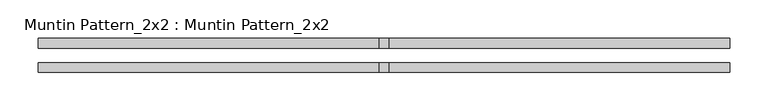
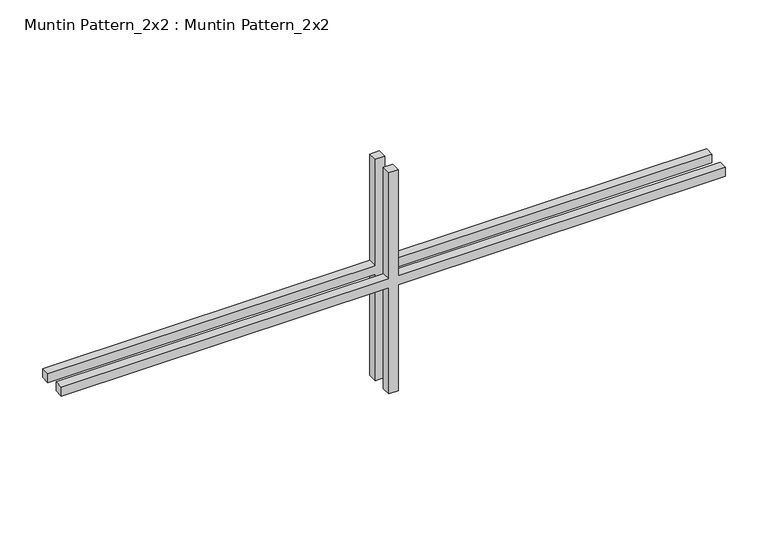
"""IFC4 building model written with IfcOpenShell, lengths in millimetres: proxy geometry, Muntin Pattern_2x2 : Muntin Pattern_2x2."""

from ifc_helpers import new_model, si_unit, frame, origin, place, context, project, spatial, polyline, outline, extrude, source, transform, mapped, element, save


def muntin_pattern_2x2_muntin_pattern_2x2_4e6d5dbc(model_context):
    return source(origin(), model_context, "Body", "SweptSolid", [
        extrude(outline(polyline([(165.1, -6.35), (165.1, -450.85), (152.4, -450.85), (152.4, -6.35), (0.0, -6.35), (0.0, 6.35), (152.4, 6.35), (152.4, 450.85), (165.1, 450.85), (165.1, 6.35), (317.5, 6.35), (317.5, -6.35), (165.1, -6.35)])), frame((0.0, 9.525, 0.0), z_axis=(0.0, 1.0, 0.0), x_axis=(0.0, 0.0, 1.0)), (0.0, 0.0, 1.0), 12.7),
        extrude(outline(polyline([(165.1, -6.35), (165.1, -450.85), (152.4, -450.85), (152.4, -6.35), (0.0, -6.35), (0.0, 6.35), (152.4, 6.35), (152.4, 450.85), (165.1, 450.85), (165.1, 6.35), (317.5, 6.35), (317.5, -6.35), (165.1, -6.35)])), frame((0.0, -22.225, 0.0), z_axis=(0.0, 1.0, 0.0), x_axis=(0.0, 0.0, 1.0)), (0.0, 0.0, 1.0), 12.7),
    ])


if __name__ == "__main__":
    model = new_model("IFC4")
    model_context = context("Model", 3, world=origin())
    ifc_project = project(units=[si_unit("LENGTHUNIT", "METRE", prefix="MILLI")], contexts=[model_context])
    site = spatial("IfcSite", under=ifc_project)
    building = spatial("IfcBuilding", under=site)
    placement = place(None, origin())
    muntin_pattern_2x2_muntin_pattern_2x2_shape = muntin_pattern_2x2_muntin_pattern_2x2_4e6d5dbc(model_context)
    element("IfcBuildingElementProxy", 1, Name="Muntin Pattern_2x2 : Muntin Pattern_2x2", ObjectType="Muntin Pattern_2x2 : Muntin Pattern_2x2", at=placement, inside=building, context=model_context, shape_type="MappedRepresentation", body=[
        mapped(muntin_pattern_2x2_muntin_pattern_2x2_shape, transform((0.0, 0.0, 0.0), x_axis=(1.0, 0.0, 0.0), y_axis=(0.0, 1.0, 0.0), z_axis=(0.0, 0.0, 1.0))),
    ])
    save(model, "model.ifc")

# Revit data of these elements
# Type "Muntin Pattern_2x2 : Muntin Pattern_2x2"
#   Width [instance default] = 4' - 0"
#   Thickness = 0' - 0 1/2"
#   Height [instance default] = 4' - 0"
#   Distance = 0' - 0 3/4"
#   Interior Material [instance default] = none
#   Exterior Material [instance default] = none
#   Default Elevation = 0
# Element 1 (IfcBuildingElementProxy, "Muntin Pattern_2x2 : Muntin Pattern_2x2")
#   Width = 2' - 11 1/2"
#   Height = 1' - 0 1/2"
#   Interior Material = Wood - Stained
#   Exterior Material = Clad - White
#   Materials on its faces: "Clad - White", "Wood - Stained"
# Materials
#   "Clad - White": class "Wood", colour RGB 242 242 238, transparency 0, Cost = 0
#   "Wood - Stained": class "Wood", colour RGB 224 178 126, transparency 0, Cost = 0
